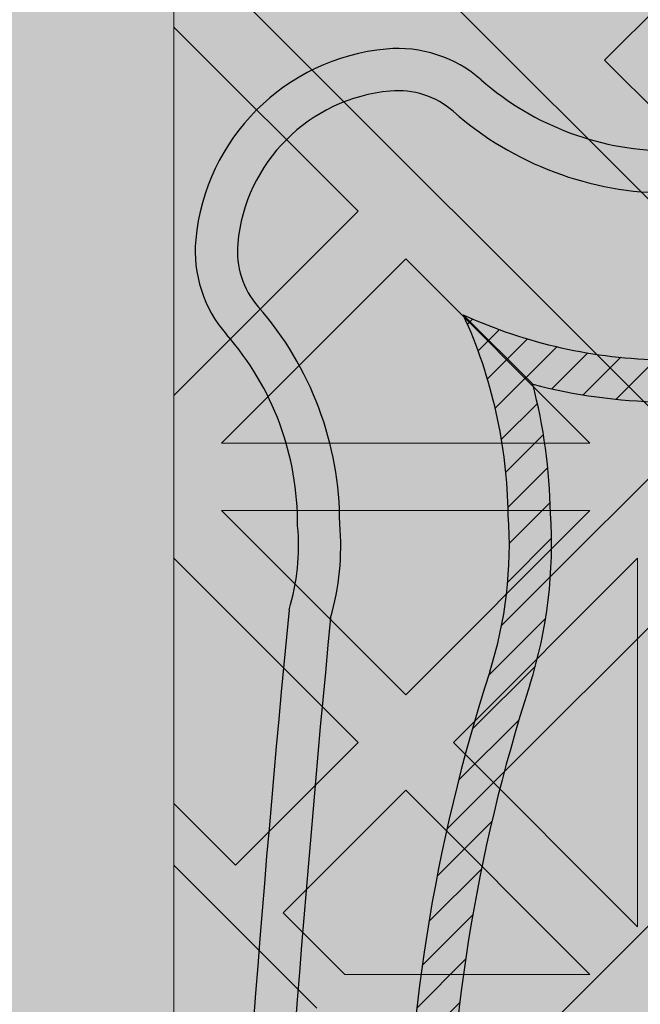
# Model space of a CAD drawing. Units: inches. Extents: x 844 to 2234, y 346 to 1084.
# Tile 58 of 93: x 1864.294 to 1866.641, y 706.48 to 710.205. Entities that reach past the tile are written whole.
import ezdxf

# ---------------------------------------------------------------- set-up
doc = ezdxf.new("R2010")
doc.units = ezdxf.units.IN
doc.header["$MEASUREMENT"] = 0
doc.layers.add('furniture', color=8, linetype='Continuous', lineweight=18)
doc.layers.add('RA-AP-01$0$INT', color=35, linetype='Continuous', lineweight=5)
doc.layers.add('RA-AP-01$0$FURN', color=3, linetype='Continuous')
doc.layers.add('RA-AP-01$0$WOOD', color=64, linetype='Continuous')

# ---------------------------------------------------------------- blocks, each defined once
blk = doc.blocks.new('A$C18D01794')
at = {"layer": 'RA-AP-01$0$INT'}
blk.add_hatch(color=256, dxfattribs=at).paths.add_polyline_path([(4.505206456958071, -7.906712009588039), (5.305206456958072, -7.906712009588039), (5.305206456958072, -7.106712009588038), (5.255206456951893, -7.106712009588036), (5.25520645694868, -7.856712009570104), (4.555206456959269, -7.856712009588616), (4.555206456956052, -7.106712009588038), (4.505206456958073, -7.106712009588038)])
h = blk.add_hatch(color=256, dxfattribs=at)
h.paths.add_polyline_path([(4.585917135068448, -7.856712009587804), (4.614201406330596, -7.856712009587056), (4.668846067270487, -7.802067348644738), (4.723490728212344, -7.856712009584164), (4.771774999457151, -7.856712009582887), (4.826419660396886, -7.80206734864072), (4.862780050090322, -7.838427738332541), (4.844495778842715, -7.856712009580965), (4.862780050090411, -7.856712009580482), (4.905206456960182, -7.814285602707865), (4.947632863832445, -7.856712009578238), (4.965917135079675, -7.856712009577755), (4.947632863831759, -7.838427738330656), (4.983993253523576, -7.802067348637219), (5.038637914464627, -7.856712009575829), (5.08692218571208, -7.856712009574554), (5.141566846649976, -7.802067348634224), (5.196211507589851, -7.856712009571666), (5.224495778822615, -7.856712009570916), (4.905206456953975, -7.537422687702283)])
h.paths.add_polyline_path([(4.895206456956031, -7.575706958950402), (4.895206456958921, -7.684996280828174), (4.840561796018589, -7.630351619890275)], flags=16)
h.paths.add_polyline_path([(4.915206456955638, -7.575706958949956), (4.969851117895509, -7.630351619887399), (4.915206456957609, -7.684996280827732)], flags=16)
h.paths.add_polyline_path([(4.826419660395175, -7.644493755514321), (4.881064321335613, -7.699138416452331), (4.771774999456703, -7.69913841645522)], flags=16)
h.paths.add_polyline_path([(4.983993253519558, -7.644493755510815), (5.038637914460456, -7.699138416449285), (4.929348592581548, -7.69913841645126)], flags=16)
h.paths.add_polyline_path([(4.881064321336025, -7.719138416452334), (4.826419660397532, -7.773783077393256), (4.771774999457062, -7.719138416455217)], flags=16)
h.paths.add_polyline_path([(4.929348592582019, -7.71913841645126), (5.038637914460982, -7.719138416449284), (4.983993253522945, -7.773783077389749)], flags=16)
h.paths.add_polyline_path([(4.895206456960191, -7.733280552075633), (4.895206456962115, -7.806001331460164), (4.876922185715016, -7.824285602708492), (4.840561796021581, -7.787925213016675)], flags=16)
h.paths.add_polyline_path([(4.915206456958487, -7.733280552075187), (4.969851117899527, -7.787925213013798), (4.933490728206909, -7.824285602708034), (4.9152064569598, -7.806001331461736)], flags=16)
h.paths.add_polyline_path([(4.757632863832376, -7.733280552079264), (4.812277524772842, -7.787925213017304), (4.757632863834348, -7.842569873958233)], flags=16)
h.paths.add_polyline_path([(4.737632863832376, -7.73328055207979), (4.737632863834348, -7.842569873958701), (4.682988202893906, -7.787925213020692)], flags=16)
h.paths.add_polyline_path([(5.05278005008503, -7.733280552072701), (5.052780050087917, -7.842569873951664), (4.998135389146995, -7.787925213013169)], flags=16)
h.paths.add_polyline_path([(5.072780050085024, -7.733280552072333), (5.127424711025931, -7.787925213010806), (5.072780050087916, -7.842569873951244)], flags=16)
h.paths.add_polyline_path([(4.935917135072783, -7.506712009583784), (5.255206456948811, -7.826001331459767), (5.255206456948932, -7.797717060211899), (5.200561796010279, -7.743072399273238), (5.255206456949403, -7.688427738334128), (5.25520645694961, -7.640143467086677), (5.200561796009787, -7.585498806146837), (5.236922185702417, -7.549138416454212), (5.255206456949919, -7.56742268770172), (5.255206456949998, -7.549138416454178), (5.212780050078687, -7.506712009583814), (5.25520645695036, -7.464285602712145), (5.255206456950438, -7.446001331464763), (5.236922185702424, -7.464285602712779), (5.200561796009796, -7.427925213020149), (5.255206456950753, -7.373280552079203), (5.25520645695096, -7.324996280834394), (5.200561796010322, -7.270351619893748), (5.255206456951428, -7.215706958952649), (5.255206456951547, -7.187422687705071)])
h.paths.add_polyline_path([(5.042988202883395, -7.42792521302065), (5.097632863823085, -7.373280552080975), (5.097632863822622, -7.482569873959883)], flags=16)
h.paths.add_polyline_path([(5.028846067259663, -7.442067348644384), (5.083490728198774, -7.496712009583504), (4.974201406321001, -7.496712009583035)], flags=16)
h.paths.add_polyline_path([(5.117632863823087, -7.37328055208089), (5.172277524762331, -7.42792521302015), (5.11763286382262, -7.482569873959851)], flags=16)
h.paths.add_polyline_path([(5.08349072819877, -7.516712009582191), (5.028846067259652, -7.571356670521302), (4.974201406320998, -7.516712009582638)], flags=16)
h.paths.add_polyline_path([(5.131774999446817, -7.35913841645716), (5.186419660386065, -7.413783077396415), (5.241064321325782, -7.359138416456712)], flags=17)
h.paths.add_polyline_path([(5.131774999446228, -7.496712009583703), (5.186419660386065, -7.442067348643883), (5.222780050079488, -7.478427738337313), (5.204495778832781, -7.496712009584014)], flags=16)
h.paths.add_polyline_path([(5.097632863822613, -7.530854145205813), (5.097632863823061, -7.640143467084723), (5.042988202883383, -7.585498806145032)], flags=16)
h.paths.add_polyline_path([(5.131774999446899, -7.339138416457162), (5.241064321325809, -7.339138416456712), (5.186419660386591, -7.284493755517479)], flags=17)
h.paths.add_polyline_path([(5.131774999446226, -7.516712009581999), (5.204495778830767, -7.516712009581702), (5.22278005007868, -7.534996280829206), (5.186419660386049, -7.571356670521828)], flags=16)
h.paths.add_polyline_path([(5.11763286382262, -7.530854145205852), (5.17227752476232, -7.585498806145562), (5.117632863823064, -7.64014346708481)], flags=16)
h.paths.add_polyline_path([(5.186419660386069, -7.599640941770585), (5.241064321325754, -7.654285602710281), (5.131774999446791, -7.654285602709814)], flags=16)
h.paths.add_polyline_path([(5.131774999446872, -7.674285602709813), (5.24106432132578, -7.674285602710282), (5.186419660386554, -7.728930263649504)], flags=16)
h.paths.add_polyline_path([(5.255206456951811, -7.126001331467467), (5.255206456951895, -7.106712009588038), (4.555206456956052, -7.106712009588038), (4.555206456956136, -7.12600133146746), (4.905206456953973, -7.476001331465289)])
h.paths.add_polyline_path([(4.983993253513404, -7.368930263651977), (4.92934859257295, -7.314285602713969), (5.03863791445186, -7.314285602711063)], flags=16)
h.paths.add_polyline_path([(4.969851117889988, -7.383072399276016), (4.915206456952556, -7.437717060215906), (4.915206456949648, -7.328427738338133)], flags=16)
h.paths.add_polyline_path([(4.929348592572535, -7.294285602713971), (4.983993253511019, -7.239640941773039), (5.038637914451496, -7.294285602711065)], flags=16)
h.paths.add_polyline_path([(5.052780050074912, -7.280143467087016), (4.998135389134438, -7.225498806148989), (5.052780050072919, -7.170854145208052)], flags=16)
h.paths.add_polyline_path([(5.07278005007491, -7.280143467086489), (5.072780050072918, -7.170854145207579), (5.127424711013374, -7.225498806145578)], flags=16)
h.paths.add_polyline_path([(4.89520645695295, -7.437717060216355), (4.840561796013067, -7.383072399278919), (4.895206456950961, -7.328427738338582)], flags=16)
h.paths.add_polyline_path([(4.915206456948365, -7.280143467090674), (4.915206456946434, -7.207422687704125), (4.933490728192729, -7.18913841645701), (4.969851117886972, -7.225498806149623)], flags=16)
h.paths.add_polyline_path([(4.881064321327021, -7.314285602715054), (4.82641966038902, -7.368930263655506), (4.771774999448108, -7.314285602717047)], flags=16)
h.paths.add_polyline_path([(4.895206456950073, -7.280143467091125), (4.840561796009022, -7.225498806152518), (4.876922185700835, -7.18913841645908), (4.895206456948749, -7.207422687706589)], flags=16)
h.paths.add_polyline_path([(4.983993253510392, -7.211356670525576), (4.947632863816944, -7.174996280833758), (4.965917135064043, -7.156712009585847), (5.038637914448995, -7.156712009584522)], flags=16)
h.paths.add_polyline_path([(4.881064321326543, -7.294285602715056), (4.771774999447578, -7.294285602717046), (4.826419660385607, -7.239640941776569)], flags=16)
h.paths.add_polyline_path([(4.905206456946447, -7.19913841645844), (4.862780050074785, -7.156712009587725), (4.947632863816685, -7.156712009586302)], flags=16)
h.paths.add_polyline_path([(5.14156684663679, -7.211356670521528), (5.086922185696452, -7.156712009583639), (5.196211507574223, -7.156712009581651)], flags=16)
h.paths.add_polyline_path([(4.8264196603837, -7.211356670529104), (4.771774999442643, -7.156712009590501), (4.8444957788276, -7.156712009588568), (4.862780050075511, -7.17499628083566)], flags=16)
h.paths.add_polyline_path([(4.812277524760289, -7.225498806153156), (4.757632863822258, -7.28014346709363), (4.757632863819352, -7.170854145214669)], flags=16)
h.paths.add_polyline_path([(4.73763286382226, -7.280143467093997), (4.682988202881349, -7.22549880615554), (4.737632863819352, -7.170854145215086)], flags=16)
h.paths.add_polyline_path([(4.723490728195188, -7.156712009591787), (4.668846067257299, -7.211356670532127), (4.614201406317417, -7.156712009594693)], flags=16)
h.paths.add_polyline_path([(4.597632863829262, -7.506712009583814), (4.555206456957951, -7.54913841645418), (4.555206456958029, -7.56742268770172), (4.573490728205535, -7.549138416454212), (4.609851117898167, -7.585498806146839), (4.555206456958338, -7.640143467086675), (4.555206456958546, -7.688427738334125), (4.60985111789767, -7.743072399273238), (4.555206456959015, -7.797717060211899), (4.555206456959138, -7.826001331459767), (4.874495778835167, -7.506712009583786), (4.5552064569564, -7.187422687705062), (4.555206456956523, -7.215706958952644), (4.609851117897629, -7.270351619893746), (4.555206456956988, -7.324996280834396), (4.555206456957198, -7.373280552079195), (4.609851117898153, -7.427925213020147), (4.573490728205528, -7.464285602712779), (4.555206456957507, -7.446001331464756), (4.555206456957585, -7.464285602712143)])
h.paths.add_polyline_path([(4.712780050085332, -7.482569873959882), (4.712780050084863, -7.373280552080972), (4.767424711024555, -7.42792521302065)], flags=16)
h.paths.add_polyline_path([(4.726922185709173, -7.496712009583504), (4.781566846648288, -7.442067348644384), (4.836211507586949, -7.496712009583033)], flags=16)
h.paths.add_polyline_path([(4.692780050085327, -7.482569873959851), (4.638135389145619, -7.427925213020149), (4.692780050084865, -7.373280552080892)], flags=16)
h.paths.add_polyline_path([(4.726922185709182, -7.516712009582191), (4.836211507586949, -7.51671200958264), (4.7815668466483, -7.571356670521304)], flags=16)
h.paths.add_polyline_path([(4.678637914461726, -7.496712009583706), (4.605917135075169, -7.496712009584014), (4.587632863828464, -7.478427738337311), (4.623993253521887, -7.442067348643881)], flags=16)
h.paths.add_polyline_path([(4.712780050085336, -7.530854145205816), (4.767424711024568, -7.585498806145034), (4.71278005008489, -7.640143467084724)], flags=16)
h.paths.add_polyline_path([(4.678637914461726, -7.516712009582001), (4.623993253521899, -7.571356670521829), (4.587632863829271, -7.534996280829206), (4.605917135077185, -7.5167120095817)], flags=16)
h.paths.add_polyline_path([(4.692780050085336, -7.530854145205848), (4.692780050084889, -7.64014346708481), (4.638135389145632, -7.585498806145562)], flags=16)
h.paths.add_polyline_path([(4.623993253521885, -7.413783077396415), (4.678637914461131, -7.359138416457161), (4.56934859258217, -7.359138416456712)], flags=17)
h.paths.add_polyline_path([(4.623993253521901, -7.599640941770568), (4.678637914461158, -7.654285602709814), (4.569348592582195, -7.654285602710281)], flags=16)
h.paths.add_polyline_path([(4.678637914461051, -7.339138416457162), (4.623993253521361, -7.284493755517479), (4.569348592582143, -7.339138416456712)], flags=17)
h.paths.add_polyline_path([(4.678637914461076, -7.674285602709813), (4.623993253521399, -7.728930263649504), (4.569348592582167, -7.674285602710281)], flags=16)
h = blk.add_hatch(color=256, dxfattribs=at)
h.paths.add_polyline_path([(4.905206456954232, -7.537422687702028), (4.874495778835232, -7.506712009583718), (4.555206456959138, -7.826001331459766), (4.555206456959269, -7.856712009588616), (4.585917135068449, -7.856712009587804)])
h.paths.add_polyline_path([(4.935917135072152, -7.506712009583152), (4.905206456953497, -7.537422687701806), (5.224495778822614, -7.856712009570917), (5.255206456948681, -7.856712009570104), (5.255206456948813, -7.826001331459768)])
h.paths.add_polyline_path([(5.255206456951549, -7.18742268770507), (5.255206456951813, -7.126001331467461), (4.905206456953563, -7.476001331465701), (4.935917135072559, -7.506712009584006)])
h.paths.add_polyline_path([(4.874495778835167, -7.506712009583785), (4.905206456953818, -7.476001331465132), (4.555206456956135, -7.126001331467458), (4.555206456956399, -7.187422687705064)])
h = blk.add_hatch(color=256, dxfattribs=at)
h.paths.add_polyline_path([(4.781566846647504, -7.442067348645805), (4.836211507586161, -7.496712009584463), (4.726922185708388, -7.496712009584918)])
h.paths.add_polyline_path([(4.836211507586161, -7.516712009584068), (4.781566846647504, -7.571356670522723), (4.726922185708388, -7.516712009583606)])
h.paths.add_polyline_path([(4.76742471102377, -7.585498806146453), (4.712780050084083, -7.640143467086137), (4.712780050084542, -7.530854145207227)])
h.paths.add_polyline_path([(4.692780050084544, -7.530854145207257), (4.692780050084084, -7.64014346708622), (4.638135389144834, -7.585498806146965)])
h.paths.add_polyline_path([(4.678637914460932, -7.516712009583407), (4.623993253521102, -7.571356670523233), (4.587632863827676, -7.53499628082981), (4.605917135074382, -7.516712009583104)])
h.paths.add_polyline_path([(4.573490728204743, -7.54913841645434), (4.60985111789737, -7.585498806146969), (4.555206456957541, -7.640143467086797), (4.555206456957237, -7.567422687701846)])
h.paths.add_polyline_path([(4.623993253521098, -7.599640941770699), (4.67863791446035, -7.654285602709951), (4.56934859258139, -7.654285602710407)])
h.paths.add_polyline_path([(4.678637914460275, -7.67428560270995), (4.623993253520583, -7.728930263649637), (4.56934859258136, -7.674285602710405)])
h.paths.add_polyline_path([(4.609851117896854, -7.743072399273369), (4.555206456958196, -7.797717060212026), (4.555206456957738, -7.688427738334254)])
h.paths.add_polyline_path([(4.597632863828475, -7.506712009583301), (4.555206456957283, -7.549138416454495), (4.555206456956805, -7.464285602712587)])
h.paths.add_polyline_path([(4.678637914460932, -7.496712009585113), (4.605917135076396, -7.496712009585417), (4.587632863828479, -7.478427738337913), (4.623993253521104, -7.442067348645284)])
h.paths.add_polyline_path([(4.692780050084091, -7.373280552082301), (4.692780050084548, -7.482569873961267), (4.638135389144834, -7.427925213021552)])
h.paths.add_polyline_path([(4.767424711023772, -7.427925213022072), (4.712780050084545, -7.48256987396129), (4.712780050084089, -7.373280552082384)])
h.paths.add_polyline_path([(4.67863791446036, -7.359138416457298), (4.623993253521105, -7.41378307739655), (4.569348592581399, -7.35913841645684)])
h.paths.add_polyline_path([(4.609851117897371, -7.427925213020278), (4.573490728204743, -7.464285602712907), (4.555206456957237, -7.446001331465401), (4.555206456957548, -7.373280552080448)])
h.paths.add_polyline_path([(4.623993253520596, -7.284493755517612), (4.67863791446028, -7.339138416457299), (4.569348592581367, -7.339138416456838)])
h.paths.add_polyline_path([(4.609851117896867, -7.270351619893878), (4.555206456957749, -7.324996280832994), (4.55520645695821, -7.21570695895522)])
h = blk.add_hatch(color=256, dxfattribs=at)
h.paths.add_polyline_path([(4.969851117891331, -7.630351619889621), (4.915206456952669, -7.575706958950966), (4.915206456952222, -7.684996280828739)])
h.paths.add_polyline_path([(4.895206456953064, -7.575706958950968), (4.840561796014413, -7.630351619889628), (4.895206456953533, -7.684996280828741)])
h.paths.add_polyline_path([(4.826419660390684, -7.644493755513362), (4.771774999451003, -7.699138416453052), (4.881064321329913, -7.699138416452587)])
h.paths.add_polyline_path([(4.881064321329884, -7.719138416452585), (4.771774999450921, -7.719138416453052), (4.82641966039018, -7.773783077392298)])
h.paths.add_polyline_path([(4.895206456953734, -7.733280552076196), (4.840561796013912, -7.787925213016031), (4.876922185707337, -7.824285602709455), (4.895206456954043, -7.806001331462747)])
h.paths.add_polyline_path([(4.862780050082808, -7.838427738332388), (4.826419660390178, -7.802067348639763), (4.771774999450351, -7.856712009579595), (4.844495778835303, -7.856712009579895)])
h.paths.add_polyline_path([(4.812277524766446, -7.787925213016036), (4.757632863827191, -7.733280552076788), (4.757632863826741, -7.842569873955747)])
h.paths.add_polyline_path([(4.737632863827191, -7.733280552076863), (4.682988202887508, -7.787925213016558), (4.737632863826743, -7.842569873955778)])
h.paths.add_polyline_path([(4.668846067263777, -7.802067348640287), (4.614201406325123, -7.856712009578949), (4.723490728202894, -7.856712009579402)])
h.paths.add_polyline_path([(4.905206456953846, -7.814285602708654), (4.862780050082654, -7.856712009579847), (4.947632863824561, -7.85671200958032)])
h.paths.add_polyline_path([(4.915206456952028, -7.733280552076195), (4.91520645695173, -7.806001331460731), (4.933490728199234, -7.824285602708648), (4.96985111789186, -7.787925213016022)])
h.paths.add_polyline_path([(5.038637914454841, -7.719138416453029), (4.929348592575874, -7.71913841645258), (4.983993253515593, -7.773783077392289)])
h.paths.add_polyline_path([(4.983993253515065, -7.644493755513352), (4.929348592575849, -7.699138416452582), (5.038637914454755, -7.699138416453031)])
h.paths.add_polyline_path([(5.052780050079843, -7.73328055207676), (4.998135389140595, -7.787925213016018), (5.052780050080309, -7.842569873955721)])
h.paths.add_polyline_path([(4.983993253516868, -7.802067348639752), (4.947632863824241, -7.838427738332383), (4.965917135071747, -7.856712009579888), (5.038637914456701, -7.856712009579572)])
h.paths.add_polyline_path([(5.127424711019533, -7.787925213016519), (5.072780050079843, -7.733280552076838), (5.07278005008031, -7.842569873955751)])
h.paths.add_polyline_path([(5.141566846643269, -7.802067348640248), (5.086922185704154, -7.85671200957937), (5.196211507581929, -7.856712009578901)])
for p, q in [((4.555206456956052, -7.106712009588036), (4.555206456959269, -7.856712009588616)), ((4.55520645695807, -7.464285602712626), (4.555206456957598, -7.549138416454534)), ((4.597632863829264, -7.506712009583814), (4.555206456957598, -7.549138416454534)), ((4.874495778835167, -7.506712009583786), (4.555206456959136, -7.826001331459769)), ((4.605917135074869, -7.516712009584017), (4.587632863829269, -7.534996280829206)), ((4.605917135076771, -7.5167120095817), (4.678637914461723, -7.516712009581999)), ((4.678637914461723, -7.516712009581999), (4.623993253521898, -7.571356670521829)), ((4.692780050085336, -7.530854145205847), (4.638135389145632, -7.585498806145562)), ((4.692780050084889, -7.64014346708481), (4.692780050085336, -7.530854145205847)), ((4.623993253521899, -7.571356670521829), (4.587632863829269, -7.534996280829206)), ((4.905206456953975, -7.537422687702283), (4.585917135071132, -7.856712009585121)), ((4.555206456958031, -7.56742268770172), (4.573490728205535, -7.549138416454212)), ((4.609851117898167, -7.585498806146839), (4.573490728205535, -7.549138416454214)), ((4.555206456958033, -7.56742268770172), (4.555206456958345, -7.640143467086671)), ((4.555206456958345, -7.640143467086671), (4.609851117898167, -7.585498806146837)), ((4.692780050084889, -7.64014346708481), (4.638135389145632, -7.585498806145562)), ((4.569348592582195, -7.654285602710281), (4.623993253521901, -7.599640941770568)), ((4.678637914461158, -7.654285602709814), (4.623993253521901, -7.599640941770568)), ((4.678637914461158, -7.654285602709814), (4.569348592582195, -7.654285602710281)), ((4.569348592582168, -7.674285602710281), (4.623993253521399, -7.728930263649504)), ((4.678637914461078, -7.674285602709813), (4.569348592582168, -7.674285602710281)), ((4.6239932535214, -7.728930263649502), (4.678637914461078, -7.674285602709813)), ((4.555206456958551, -7.68842773833413), (4.60985111789767, -7.743072399273238)), ((4.682988202893908, -7.78792521302069), (4.737632863832376, -7.733280552079792)), ((4.555206456959017, -7.797717060211899), (4.60985111789767, -7.743072399273238)), ((4.737632863834348, -7.842569873958701), (4.682988202893906, -7.787925213020692))]:
    blk.add_line(p, q, dxfattribs=at)
blk = doc.blocks.new('A$C32926AE1')
at = {"layer": 'RA-AP-01$0$WOOD'}
h = blk.add_hatch(color=256, dxfattribs=at)
h.dxf.hatch_style = 1
h.paths.add_polyline_path([(5.157430609644524, 4.573483066760929, -0.1009492694046607), (5.155401577623758, 4.593365984175333, -0.1842662638101597), (5.172249623284174, 4.638795604568598, 0.2056608120311276), (5.179560981299304, 4.661316324430096, 0.3614336704623542), (5.134352340494423, 4.706524965234944, 0.2056608120311297), (5.111831620632933, 4.699213607219793, -0.1842662638101113), (5.066402000239693, 4.682365561559342, -0.1055311479399994), (5.045656153913092, 4.68467289944697, 0.1567636581983829), (4.763886414745334, 4.684672899446966, -0.1055311479399895), (4.743140568418733, 4.68236556155934, -0.1842662638100833), (4.6977109480255, 4.69921360721979, 0.2056608120302612), (4.675190228164109, 4.706524965234949, 0.3614336704708441), (4.629981587358889, 4.66131632442871, 0.2056608120245944), (4.637292945374126, 4.638795604567974, -0.1842662638101024), (4.654140991034615, 4.59336598417475, -0.1009492694055169), (4.652111959013835, 4.573483066760181, 0.021410119221476), (4.629748025606143, 4.156712009541676, 0.0214101192214795), (4.652111959013809, 3.739940952323101, -0.1009492694059586), (4.654140991034615, 3.720058034908448, -0.1842662638100975), (4.637292945374126, 3.674628414515226, 0.2056608120245705), (4.629981587358889, 3.652107694654492, 0.3614336704708879), (4.675190228164113, 3.606899053848249, 0.2056608120302384), (4.697710948025501, 3.614210411863408, -0.1842662638100995), (4.743140568418738, 3.63105845752386, -0.1055311479402541), (4.763886414745388, 3.628751119636215, 0.1567636581983776), (5.045656153913137, 3.628751119636244, -0.1055311479397538), (5.066402000239692, 3.631058457523857, -0.1842662638101067), (5.111831620632931, 3.614210411863407, 0.2056608120310924), (5.134352340494417, 3.606899053848256, 0.3614336704624001), (5.179560981299307, 3.652107694653103, 0.2056608120311314), (5.172249623284175, 3.6746284145146, -0.1842662638101402), (5.155401577623758, 3.72005803490786, -0.1009492694051366), (5.15743060964455, 3.739940952322354, 0.0214101192215073), (5.179794543052287, 4.156712009541468, 0.0214101192215252)])
h.paths.add_polyline_path([(4.639748609479751, 4.156712009541513, 0.0213537860821624), (4.661970494867118, 3.741887061152232, -0.094075836301374), (4.664143710413708, 3.7196126951003, -0.1824818158568985), (4.644813765429836, 3.668037719127816, 0.2056608120245319), (4.639939526753007, 3.653023905887301, 0.3614336704710246), (4.676106439397173, 3.616856993242342, 0.2056608120302234), (4.691120252638095, 3.621731231919122, -0.1824818158602558), (4.742695228611606, 3.641061176902986, -0.1029891339458722), (4.766991894714349, 3.638256818950944, 0.156709409989566), (5.042550673941472, 3.638256818950105, -0.102989133958497), (5.066847340047078, 3.641061176902949, -0.1824818158594995), (5.118422316020358, 3.621731231919103, 0.2056608120311416), (5.133436129261316, 3.616856993242346, 0.3614336704621468), (5.169603041905217, 3.653023905886178, 0.2056608120310986), (5.164728803228477, 3.668037719127177, -0.1824818158565612), (5.145398858244737, 3.719612695099578, -0.0940758363009313), (5.147572073791232, 3.741887061151398, 0.0213537860822023), (5.169793959178681, 4.156712009541451, 0.0213537860822226), (5.147572073791203, 4.571536957931898, -0.0940758363005034), (5.145398858244737, 4.59381132398362, -0.1824818158565587), (5.164728803228476, 4.645386299956021, 0.2056608120311045), (5.169603041905216, 4.66040011319702, 0.3614336704621845), (5.133436129261313, 4.696567025840856, 0.2056608120310773), (5.118422316020359, 4.691692787164098, -0.182481815859508), (5.066847340047078, 4.67236284218025, -0.1029891339584606), (5.04255067394148, 4.675167200133092, 0.156709409989566), (4.766991894714357, 4.675167200132257, -0.1029891339458842), (4.742695228611611, 4.672362842180213, -0.1824818158602725), (4.691120252638095, 4.691692787164077, 0.2056608120302152), (4.676106439397174, 4.696567025840858, 0.3614336704710363), (4.639939526753005, 4.660400113195899, 0.2056608120245495), (4.644813765429837, 4.645386299955384, -0.1824818158568934), (4.664143710413708, 4.593811323982902, -0.0940758363009187), (4.661970494867149, 4.571536957931074, 0.021353786082177)], flags=16)
h.paths.add_polyline_path([(5.129794543052235, 4.432167055276933, -0.0141661062790638), (5.130152669293814, 4.156927903047693, -0.0141661062790647), (5.129794543052234, 3.881688750818433, -0.0785247771143638), (5.10979738006795, 3.755143611847103, 0.0945969212073497), (5.105408519571111, 3.717898134952927, 0.1043170707844957), (5.116074640131521, 3.670385395016088, 0.1043170707864965), (5.068561900193738, 3.681051515576561, 0.09459692119553), (5.031316423304057, 3.676662655080835, -0.1580239521427272), (4.778226145355827, 3.676662655080367, 0.0945969211986668), (4.740980668464973, 3.681051515576592, 0.1043170707882822), (4.693467928526415, 3.670385395015844, 0.1043170707867916), (4.704134049087309, 3.717898134953662, 0.0945969211972894), (4.69974518859162, 3.755143611844042, -0.0785247771163196), (4.679748025606343, 3.881688750818406, -0.0141661062790663), (4.679389899364763, 4.156927903047693, -0.0141661062790672), (4.679748025606343, 4.432167055276998, -0.0785247771163064), (4.699745188591625, 4.55871219425134, 0.094596921197333), (4.704134049087308, 4.595957671141738, 0.1043170707867205), (4.693467928526416, 4.643470411079523, 0.1043170707882628), (4.740980668464965, 4.632804290518776, 0.0945969211988114), (4.778226145355874, 4.637193151015016, -0.158023952142669), (5.031316423304015, 4.637193151014546, 0.0945969211956361), (5.068561900193736, 4.632804290518806, 0.1043170707864979), (5.11607464013152, 4.643470411079278, 0.1043170707844617), (5.105408519571112, 4.595957671142455, 0.0945969212074597), (5.109797380067959, 4.558712194248236, -0.0785247771143467)], flags=0)
h.paths.add_polyline_path([(5.119794532311105, 4.432259799204851, -0.0142000800617244), (5.120156169157484, 4.156927903047701, -0.0142000800617277), (5.119794532311105, 3.881596006890482, -0.0784894509520253), (5.100273383573699, 3.758192358677797, 0.0940138827242913), (5.095413455884425, 3.717477693979438, 0.0606271852308753), (5.099615656341024, 3.686844378806616, 0.0606271852322524), (5.068982341167493, 3.691046579263239, 0.0940138827010453), (5.028267676478798, 3.686186651576848, -0.1580706864508061), (4.781274892180912, 3.686186651576435, 0.0940138827026903), (4.740560227491556, 3.691046579263279, 0.0606271852339895), (4.709926912317155, 3.686844378806508, 0.0606271852329405), (4.714129112773991, 3.717477693980356, 0.094013882701304), (4.709269185087677, 3.758192358669163, -0.0784894509577193), (4.689748036347473, 3.881596006890469, -0.014200080061729), (4.689386399501094, 4.156927903047709, -0.0142000800617217), (4.689748036347473, 4.432259799204808, -0.078489450957724), (4.709269185087651, 4.555663447426125, 0.0940138827014585), (4.714129112773992, 4.596378112114996, 0.0606271852329731), (4.709926912317154, 4.62701142728886, 0.0606271852340196), (4.74056022749157, 4.622809226832087, 0.0940138827024997), (4.781274892180847, 4.627669154518912, -0.1580706864508359), (5.028267676478777, 4.627669154518526, 0.0940138827010946), (5.068982341167492, 4.622809226832129, 0.060627185232254), (5.099615656341024, 4.627011427288751, 0.0606271852308727), (5.095413455884425, 4.59637811211593, 0.0940138827241088), (5.100273383573675, 4.555663447417647, -0.0784894509520978)], flags=0)
h.paths.add_polyline_path([(5.06978912287499, 4.430218106756144, -0.014241683694547), (5.070173729147532, 4.156927903047672, -0.0142416836945458), (5.06978912287499, 3.883637699339223, -0.0800609523125196), (5.052662118612511, 3.773463122773442, 0.0526421978001116), (5.04590916754064, 3.740550867606997, 0.0526421977992423), (5.012996912374707, 3.73379791653534, -0.1583028414718258), (4.796545656286308, 3.73379791653451, 0.0526421978034211), (4.763633401117837, 3.740550867607021, 0.0526421978018622), (4.756880450045755, 3.773463122774558, -0.0800609523117106), (4.739753445783639, 3.883637699339268, -0.0142416836945435), (4.739368839511098, 4.156927903047671, -0.0142416836945477), (4.739753445783639, 4.430218106756155, -0.0800609523116345), (4.75688045004574, 4.540392683320762, 0.052642197801941), (4.763633401117837, 4.573304938488346, 0.0526421978035071), (4.796545656286361, 4.580057889560873, -0.1583028414717561), (5.012996912374669, 4.580057889560039, 0.0526421977993048), (5.04590916754064, 4.57330493848837, 0.0526421978002057), (5.052662118612529, 4.540392683321868, -0.080060952312477)], flags=0)
h.paths.add_polyline_path([(5.049789715110557, 4.43038092723357, -0.0143097550741839), (5.05018085590259, 4.156927903047715, -0.0143097550741854), (5.049789715110558, 3.883474878861827, -0.0800685599149176), (5.03362098255317, 3.779581877367999, 0.0306258898956367), (5.028241146483733, 3.758218888663947, 0.0306258898977031), (5.006878157778253, 3.75283905259408, -0.1583983521624096), (4.802664410878162, 3.752839052594731, 0.0306258898946014), (4.781301422174808, 3.758218888663924, 0.0306258898967912), (4.775921586105202, 3.779581877368794, -0.080068559914251), (4.759752853548071, 3.883474878861786, -0.0143097550741854), (4.759361712756037, 4.156927903047671, -0.0143097550741854), (4.759752853548071, 4.430380927233557, -0.0800685599142479), (4.775921586105193, 4.534273928726546, 0.0306258898968306), (4.781301422174808, 4.555636917431444, 0.0306258898945754), (4.802664410878143, 4.561016753500631, -0.1583983521624168), (5.006878157778244, 4.561016753501291, 0.0306258898977177), (5.028241146483733, 4.555636917431421, 0.0306258898958182), (5.03362098255321, 4.534273928727244, -0.080068559914796)], flags=0)
h.paths.add_polyline_path([(4.999766070382627, 4.428171244713864, -0.0143443147609634), (5.000198441819402, 4.156927903047689, -0.0143443147609612), (4.999766070382627, 3.885684561381556, -0.0784641635803329), (4.987356730658798, 3.799103304488872, -0.1506053783831347), (4.822185837999821, 3.79910330448882, -0.0784641635803318), (4.809776498276007, 3.885684561381509, -0.014344314760963), (4.809344126839227, 4.156927903047677, -0.0143443147609645), (4.809776498276007, 4.428171244713873, -0.0784641635803192), (4.822185837999822, 4.514752501606549, -0.1506053783831338), (4.987356730658798, 4.514752501606494, -0.078464163580285)], flags=0)
h.paths.add_polyline_path([(4.979755254238824, 4.42764379880488, -0.0143772539198268), (4.980205517789977, 4.156927903047693, -0.0143772539198275), (4.979755254238824, 3.886212007290489, -0.0689242507424422), (4.971183264704897, 3.815276770442801, -0.1296645318904179), (4.838359303953726, 3.815276770442746, -0.0689242507424186), (4.829787314419809, 3.886212007290419, -0.0143772539198292), (4.829337050868653, 4.156927903047653, -0.0143772539198325), (4.829787314419809, 4.427643798804946, -0.0689242507424211), (4.838359303953725, 4.498579035652621, -0.1296645318904187), (4.971183264704897, 4.498579035652565, -0.0689242507424401)], flags=0)
h = blk.add_hatch(color=256, dxfattribs=at)
h.dxf.hatch_style = 1
h.paths.add_polyline_path([(5.145398858244737, 4.59381132398362, -0.1824818158565616), (5.164728803228476, 4.645386299956021, 0.2056608120311045), (5.169603041905216, 4.66040011319702, 0.3614336704621845), (5.133436129261313, 4.696567025840856, 0.2056608120310773), (5.118422316020359, 4.691692787164098, -0.182481815859508), (5.066847340047078, 4.67236284218025, -0.1029891339584606), (5.04255067394148, 4.675167200133092, 0.156709409989566), (4.766991894714357, 4.675167200132257, -0.1029891339458842), (4.742695228611611, 4.672362842180213, -0.1824818158602725), (4.691120252638095, 4.691692787164077, 0.2056608120302152), (4.676106439397174, 4.696567025840858, 0.3614336704710363), (4.639939526753005, 4.660400113195899, 0.2056608120245495), (4.644813765429837, 4.645386299955384, -0.1824818158568934), (4.664143710413708, 4.593811323982902, -0.0940758363009187), (4.661970494867149, 4.571536957931074, 0.0213537860821772), (4.639748609479751, 4.156712009541507, 0.0213537860821625), (4.661970494867119, 3.741887061152226, -0.0940758363013071), (4.664143710413708, 3.719612695100309, -0.1824818158569294), (4.644813765429836, 3.668037719127816, 0.2056608120245319), (4.639939526753007, 3.653023905887301, 0.3614336704710246), (4.676106439397173, 3.616856993242342, 0.2056608120302234), (4.691120252638095, 3.621731231919122, -0.1824818158602558), (4.742695228611606, 3.641061176902986, -0.1029891339458722), (4.766991894714349, 3.638256818950944, 0.156709409989566), (5.042550673941472, 3.638256818950105, -0.102989133958497), (5.066847340047078, 3.641061176902949, -0.1824818158594995), (5.118422316020358, 3.621731231919103, 0.2056608120311416), (5.133436129261316, 3.616856993242346, 0.3614336704621468), (5.169603041905217, 3.653023905886178, 0.2056608120310986), (5.164728803228477, 3.668037719127177, -0.1824818158565612), (5.145398858244737, 3.719612695099578, -0.0940758363009313), (5.147572073791232, 3.741887061151398, 0.0213537860822023), (5.169793959178681, 4.156712009541451, 0.0213537860822226), (5.147572073791203, 4.571536957931898, -0.0940758363004996)])
h.paths.add_polyline_path([(5.109797380067958, 4.55871219424824, -0.0785247771143472), (5.129794543052234, 4.432167055276936, -0.0141661062790644), (5.130152669293814, 4.156927903047685, -0.014166106279066), (5.129794543052234, 3.881688750818401, -0.0785247771143517), (5.109797380067946, 3.755143611847092, 0.0945969212073132), (5.105408519571111, 3.717898134952929, 0.1043170707844995), (5.116074640131521, 3.670385395016088, 0.1043170707864965), (5.068561900193738, 3.681051515576561, 0.09459692119553), (5.031316423304057, 3.676662655080835, -0.1580239521427272), (4.778226145355827, 3.676662655080367, 0.0945969211986668), (4.740980668464973, 3.681051515576592, 0.1043170707882822), (4.693467928526415, 3.670385395015844, 0.1043170707867916), (4.704134049087309, 3.717898134953662, 0.0945969211972894), (4.69974518859162, 3.755143611844042, -0.0785247771163196), (4.679748025606343, 3.881688750818406, -0.0141661062790663), (4.679389899364763, 4.156927903047693, -0.0141661062790672), (4.679748025606343, 4.432167055276998, -0.0785247771163064), (4.699745188591625, 4.55871219425134, 0.094596921197333), (4.704134049087308, 4.595957671141738, 0.1043170707867205), (4.693467928526416, 4.643470411079523, 0.1043170707882628), (4.740980668464965, 4.632804290518776, 0.0945969211988114), (4.778226145355874, 4.637193151015016, -0.158023952142669), (5.031316423304015, 4.637193151014546, 0.0945969211956361), (5.068561900193736, 4.632804290518806, 0.1043170707864979), (5.11607464013152, 4.643470411079278, 0.1043170707844617), (5.105408519571112, 4.595957671142455, 0.0945969212074504)], flags=16)
h.paths.add_polyline_path([(5.100273383573655, 4.55566344741771, -0.0784894509521388), (5.119794532311105, 4.432259799204852, -0.0142000800617252), (5.120156169157484, 4.156927903047686, -0.014200080061726), (5.119794532311105, 3.881596006890502, -0.0784894509520446), (5.100273383573696, 3.758192358677786, 0.0940138827242721), (5.095413455884425, 3.717477693979436, 0.0606271852308692), (5.099615656341024, 3.686844378806616, 0.0606271852322522), (5.068982341167493, 3.691046579263239, 0.0940138827010453), (5.028267676478798, 3.686186651576848, -0.1580706864508061), (4.781274892180912, 3.686186651576435, 0.0940138827026903), (4.740560227491556, 3.691046579263279, 0.0606271852339895), (4.709926912317155, 3.686844378806508, 0.0606271852329405), (4.714129112773991, 3.717477693980356, 0.094013882701304), (4.709269185087677, 3.758192358669163, -0.0784894509577193), (4.689748036347473, 3.881596006890469, -0.014200080061729), (4.689386399501094, 4.156927903047709, -0.0142000800617217), (4.689748036347473, 4.432259799204808, -0.078489450957724), (4.709269185087651, 4.555663447426125, 0.0940138827014585), (4.714129112773992, 4.596378112114996, 0.0606271852329731), (4.709926912317154, 4.62701142728886, 0.0606271852340196), (4.74056022749157, 4.622809226832087, 0.0940138827024997), (4.781274892180847, 4.627669154518912, -0.1580706864508359), (5.028267676478777, 4.627669154518526, 0.0940138827010946), (5.068982341167492, 4.622809226832129, 0.060627185232254), (5.099615656341024, 4.627011427288751, 0.0606271852308727), (5.095413455884425, 4.59637811211593, 0.094013882723957)], flags=0)
h.paths.add_polyline_path([(5.04590916754064, 4.57330493848837, 0.0526421978002057), (5.052662118612529, 4.540392683321868, -0.0800609523124783), (5.06978912287499, 4.430218106756142, -0.0142416836945469), (5.070173729147532, 4.156927903047672, -0.0142416836945458), (5.06978912287499, 3.883637699339223, -0.0800609523125196), (5.052662118612511, 3.773463122773442, 0.0526421978001116), (5.04590916754064, 3.740550867606997, 0.0526421977992423), (5.012996912374707, 3.73379791653534, -0.1583028414718258), (4.796545656286308, 3.73379791653451, 0.0526421978034211), (4.763633401117837, 3.740550867607021, 0.0526421978018622), (4.756880450045755, 3.773463122774558, -0.0800609523117106), (4.739753445783639, 3.883637699339268, -0.0142416836945435), (4.739368839511098, 4.156927903047671, -0.0142416836945477), (4.739753445783639, 4.430218106756155, -0.0800609523116345), (4.75688045004574, 4.540392683320762, 0.052642197801941), (4.763633401117837, 4.573304938488346, 0.0526421978035071), (4.796545656286361, 4.580057889560873, -0.1583028414717561), (5.012996912374669, 4.580057889560039, 0.0526421977993048)], flags=0)
h.paths.add_polyline_path([(5.028241146483733, 4.555636917431422, 0.0306258898956949), (5.033620982553182, 4.534273928727329, -0.0800685599148649), (5.049789715110557, 4.430380927233569, -0.0143097550741839), (5.05018085590259, 4.156927903047715, -0.0143097550741854), (5.049789715110558, 3.883474878861827, -0.0800685599149176), (5.03362098255317, 3.779581877367999, 0.0306258898956367), (5.028241146483733, 3.758218888663947, 0.0306258898977031), (5.006878157778253, 3.75283905259408, -0.1583983521624096), (4.802664410878162, 3.752839052594731, 0.0306258898946014), (4.781301422174808, 3.758218888663924, 0.0306258898967912), (4.775921586105202, 3.779581877368794, -0.080068559914251), (4.759752853548071, 3.883474878861786, -0.0143097550741854), (4.759361712756037, 4.156927903047671, -0.0143097550741854), (4.759752853548071, 4.430380927233557, -0.0800685599142479), (4.775921586105193, 4.534273928726546, 0.0306258898968306), (4.781301422174808, 4.555636917431444, 0.0306258898945754), (4.802664410878143, 4.561016753500631, -0.1583983521624168), (5.006878157778244, 4.561016753501291, 0.0306258898977174)], flags=0)
h.paths.add_polyline_path([(4.987356730658798, 4.514752501606494, -0.0784641635803018), (4.999766070382627, 4.428171244713845, -0.0143443147609637), (5.000198441819402, 4.156927903047665, -0.0143443147609622), (4.999766070382628, 3.885684561381514, -0.0784641635802952), (4.987356730658797, 3.799103304488872, -0.1506053783831338), (4.822185837999821, 3.799103304488819, -0.0784641635803342), (4.809776498276007, 3.885684561381512, -0.0143443147609628), (4.809344126839227, 4.156927903047676, -0.0143443147609646), (4.809776498276007, 4.428171244713873, -0.0784641635803192), (4.822185837999822, 4.514752501606549, -0.1506053783831338)], flags=0)
h.paths.add_polyline_path([(4.971183264704897, 4.498579035652566, -0.0689242507424384), (4.979755254238824, 4.427643798804883, -0.0143772539198276), (4.980205517789977, 4.15692790304768, -0.0143772539198258), (4.979755254238823, 3.88621200729051, -0.0689242507424628), (4.971183264704897, 3.815276770442801, -0.129664531890417), (4.838359303953726, 3.815276770442746, -0.0689242507424186), (4.829787314419809, 3.886212007290419, -0.0143772539198292), (4.829337050868653, 4.156927903047653, -0.0143772539198325), (4.829787314419809, 4.427643798804946, -0.0689242507424211), (4.838359303953725, 4.498579035652621, -0.1296645318904187)], flags=0)
h = blk.add_hatch(dxfattribs=at)
h.set_pattern_fill('ANSI31', color=256, scale=0.05, style=0)
h.set_pattern_definition([(45, (0, 0), (-0.0044194173824159, 0.0044194173824159), [])])
h.paths.add_polyline_path([(5.130152669293814, 4.156927903047704, 0.0141661062790657), (5.129794543052234, 4.432167055276982, 0.0777827904001433), (5.110168979996553, 4.557559993161921, -0.0976515123401879), (5.105408519571111, 4.595957671142454, -0.1043170707844687), (5.116074640131522, 4.64347041107928), (5.099615656341024, 4.627011427288751, 0.0606271852308727), (5.095413455884425, 4.59637811211593, 0.0940138827241088), (5.100273383573675, 4.555663447417647, -0.0784894509520972), (5.119794532311105, 4.432259799204852, -0.0142000800617252), (5.120156169157484, 4.156927903047686, -0.014200080061726), (5.119794532311105, 3.881596006890502, -0.0784894509520446), (5.100273383573696, 3.758192358677786, 0.0940138827242721), (5.095413455884425, 3.717477693979436, 0.0606271852308692), (5.099615656341024, 3.686844378806616), (5.116074640131519, 3.67038539501609, -0.1043170707844594), (5.105408519571112, 3.717898134952912, -0.0976515123401594), (5.11016897999655, 3.756295812933435, 0.0777827904001654), (5.129794543052234, 3.881688750818409, 0.0141661062790665)])
h.paths.add_polyline_path([(5.030164222210597, 3.676291055149937, -0.0976515123472002), (5.068561900193739, 3.681051515576561, -0.1043170707864927), (5.116074640131521, 3.670385395016088), (5.099615656341024, 3.686844378806616, 0.0606271852322522), (5.068982341167493, 3.691046579263239, 0.0940138827010453), (5.028267676478798, 3.686186651576848, -0.1580706864508061), (4.781274892180912, 3.686186651576435, 0.0940138827026903), (4.740560227491556, 3.691046579263279, 0.0606271852339913), (4.709926912317154, 3.686844378806508), (4.693467928526416, 3.670385395015845, -0.1043170707882796), (4.740980668464973, 3.681051515576592, -0.0976515123427246), (4.779378346446416, 3.676291055150394, 0.156512506893803)])
h.paths.add_polyline_path([(4.689748036347473, 3.881596006890472, -0.014200080061729), (4.689386399501094, 4.156927903047712, -0.0142000800617195), (4.689748036347473, 4.432259799204768, -0.078489450957742), (4.709269185087648, 4.555663447426114, 0.0940138827014821), (4.714129112773992, 4.596378112114995, 0.0606271852329748), (4.709926912317154, 4.62701142728886), (4.693467928526414, 4.643470411079524, -0.1043170707867939), (4.704134049087309, 4.595957671141706, -0.09765151234893), (4.699373588660725, 4.557559993157876, 0.0777827903975372), (4.679748025606343, 4.432167055276987, 0.0141661062790675), (4.679389899364763, 4.156927903047675, 0.0141661062790641), (4.679748025606343, 3.88168875081843, 0.0777827903975637), (4.699373588660724, 3.756295812937497, -0.0976515123490278), (4.704134049087308, 3.717898134953629, -0.1043170707867196), (4.693467928526416, 3.670385395015845), (4.709926912317155, 3.686844378806508, 0.0606271852329413), (4.714129112773991, 3.717477693980357, 0.0940138827013084), (4.709269185087676, 3.758192358669166, -0.0784894509577192)])
h.paths.add_polyline_path([(4.779378346446434, 4.63756475094498, -0.0976515123427943), (4.740980668464964, 4.632804290518776, -0.1043170707882609), (4.693467928526416, 4.643470411079523), (4.709926912317154, 4.62701142728886, 0.0606271852340196), (4.74056022749157, 4.622809226832087, 0.0940138827024997), (4.781274892180847, 4.627669154518912, -0.1580706864508359), (5.028267676478777, 4.627669154518526, 0.0940138827010946), (5.068982341167492, 4.622809226832129, 0.060627185232254), (5.099615656341024, 4.627011427288751), (5.116074640131521, 4.643470411079279, -0.1043170707865022), (5.068561900193735, 4.632804290518806, -0.0976515123475899), (5.030164222210446, 4.637564750945479, 0.1565125068936924)])
h = blk.add_hatch(dxfattribs=at)
h.set_pattern_fill('ANSI32', color=256, scale=0.2, style=0)
h.set_pattern_definition([(45, (0, 0), (-0.0530330085889911, 0.0530330085889911), []), (45, (0.035355339, 0), (-0.0530330085889911, 0.0530330085889911), [])])
h.paths.add_polyline_path([(5.119794532311105, 4.432259799204823, 0.0777015974868765), (5.10065834347252, 4.554469821747928, -0.0968902511992216), (5.095413455884425, 4.596378112115931, -0.060627185230871), (5.099615656341024, 4.627011427288751, -0.060627185232254), (5.068982341167492, 4.622809226832129, -0.0968902512198245), (5.027074050790956, 4.628054114423209, 0.1564657949319105), (4.782468517866163, 4.628054114422785, -0.0968902512152247), (4.740560227491555, 4.622809226832088, -0.0606271852339878), (4.709926912317155, 4.627011427288859, -0.0606271852329413), (4.714129112773991, 4.596378112115011, -0.0968902512205338), (4.708884225182929, 4.554469821738175, 0.0777015974804443), (4.689748036347473, 4.43225979920482, 0.0142000800617215), (4.689386399501094, 4.156927903047726, 0.0142000800617273), (4.689748036347473, 3.88159600689052, 0.077701597480541), (4.708884225182985, 3.759385984357019, -0.096890251220082), (4.714129112773992, 3.717477693980371, -0.0606271852329731), (4.709926912317154, 3.686844378806507, -0.060627185233988), (4.740560227491554, 3.691046579263279, -0.0968902512152569), (4.782468517866175, 3.685801691672578, 0.1564657949319236), (5.027074050790988, 3.685801691672169, -0.0968902512197451), (5.068982341167491, 3.691046579263239, -0.0606271852322557), (5.099615656341024, 3.686844378806616, -0.0606271852308727), (5.095413455884425, 3.717477693979438, -0.0968902511991229), (5.100658343472507, 3.7593859843474, 0.0777015974868745), (5.119794532311105, 3.8815960068905, 0.014200080061726), (5.120156169157484, 4.156927903047685, 0.0142000800617238)])
h.paths.add_polyline_path([(5.070173729147531, 4.156927903047684, -0.0142416836945481), (5.06978912287499, 3.883637699339191, -0.0800609523125107), (5.052662118612505, 3.773463122773424, 0.0526421978000811), (5.04590916754064, 3.740550867606997, 0.0526421977993214), (5.012996912374658, 3.733797916535325, -0.1583028414717916), (4.796545656286304, 3.733797916534512, 0.0526421978034138), (4.763633401117837, 3.740550867607021, 0.0526421978018622), (4.756880450045755, 3.773463122774558, -0.0800609523117106), (4.739753445783639, 3.883637699339268, -0.0142416836945435), (4.739368839511098, 4.156927903047671, -0.0142416836945477), (4.739753445783639, 4.430218106756155, -0.0800609523116345), (4.75688045004574, 4.540392683320762, 0.052642197801941), (4.763633401117837, 4.573304938488346, 0.0526421978035071), (4.796545656286361, 4.580057889560873, -0.1583028414717561), (5.012996912374669, 4.580057889560039, 0.0526421977993048), (5.04590916754064, 4.57330493848837, 0.0526421978002057), (5.052662118612529, 4.540392683321868, -0.0800609523124783), (5.06978912287499, 4.430218106756142, -0.0142416836945463)], flags=16)
h.paths.add_polyline_path([(5.050180855902591, 4.156927903047686, -0.0143097550741856), (5.049789715110558, 3.883474878861795, -0.0800685599148126), (5.033620982553202, 3.7795818773681, 0.0306258898957837), (5.028241146483733, 3.758218888663947, 0.0306258898977031), (5.006878157778253, 3.75283905259408, -0.1583983521624096), (4.802664410878162, 3.752839052594731, 0.0306258898946014), (4.781301422174808, 3.758218888663924, 0.0306258898967912), (4.775921586105202, 3.779581877368794, -0.080068559914251), (4.759752853548071, 3.883474878861786, -0.0143097550741854), (4.759361712756037, 4.156927903047671, -0.0143097550741854), (4.759752853548071, 4.430380927233557, -0.0800685599142479), (4.775921586105193, 4.534273928726546, 0.0306258898968306), (4.781301422174808, 4.555636917431444, 0.0306258898945754), (4.802664410878143, 4.561016753500631, -0.1583983521624168), (5.006878157778244, 4.561016753501291, 0.0306258898977177), (5.028241146483733, 4.555636917431421, 0.0306258898958182), (5.03362098255321, 4.534273928727244, -0.0800685599147973), (5.049789715110557, 4.430380927233568, -0.0143097550741854)], flags=0)
h.paths.add_polyline_path([(5.000198441819402, 4.15692790304769, -0.0143443147609622), (4.999766070382627, 3.885684561381539, -0.0784641635803169), (4.987356730658798, 3.799103304488873, -0.1506053783831347), (4.822185837999821, 3.79910330448882, -0.0784641635803318), (4.809776498276007, 3.885684561381509, -0.014344314760963), (4.809344126839227, 4.156927903047677, -0.0143443147609645), (4.809776498276007, 4.428171244713873, -0.0784641635803192), (4.822185837999822, 4.514752501606549, -0.1506053783831338), (4.987356730658798, 4.514752501606494, -0.0784641635803018), (4.999766070382627, 4.428171244713845, -0.0143443147609624)], flags=0)
h.paths.add_polyline_path([(4.980205517789976, 4.156927903047707, -0.0143772539198295), (4.979755254238824, 3.886212007290466, -0.06892425074242), (4.971183264704897, 3.815276770442801, -0.129664531890417), (4.838359303953726, 3.815276770442746, -0.0689242507424186), (4.829787314419809, 3.886212007290419, -0.0143772539198292), (4.829337050868653, 4.156927903047653, -0.0143772539198325), (4.829787314419809, 4.427643798804946, -0.0689242507424211), (4.838359303953725, 4.498579035652621, -0.1296645318904187), (4.971183264704897, 4.498579035652565, -0.0689242507424418), (4.979755254238824, 4.427643798804878, -0.0143772539198259)], flags=0)
blk.add_line((4.709926912317154, 4.62701142728886), (4.693467928526416, 4.643470411079523), dxfattribs=at)
blk.add_line((4.709926912317154, 4.62701142728886), (4.693467928526416, 4.643470411079523), dxfattribs=at)
for centre, radius, start, end in [((4.679771284329349, 4.656735268264593), 0.0499999999998897, 95.25687599443106, 174.7431240064049), ((4.67793886186326, 4.676651147052671), 0.0299999999999992, 48.77105092035662, 95.25687599427984), ((4.742507915094499, 4.750332633143934), 0.0679700159630274, 228.7710509203537, 270.5333070513671), ((4.679771284329334, 4.656735268264609), 0.0399999999998732, 95.25687599445018, 174.7431240064249), ((4.67793886186326, 4.676651147052671), 0.0199999999999984, 48.77105092035742, 95.25687599428184), ((4.742507915094546, 4.750332633143919), 0.0779700159630467, 228.7710509203206, 270.1376463011373), ((4.659855405541232, 4.658567690730234), 0.0300000000000005, 174.7431240062535, 221.2289490796905), ((4.65985540554127, 4.658567690730245), 0.0200000000000369, 174.7431240062188, 221.2289490796444), ((4.586173919450017, 4.593998637498934), 0.077970015963029, 359.8623536996133, 41.22894907969008), ((4.586173919450015, 4.5944304245111), 0.1179700159630316, 0.7417751874182703, 24.56332695026347), ((4.742507915094493, 4.750764420156106), 0.1179700159630538, 245.436673049926, 269.258224813113), ((4.586173919450019, 4.593998637498935), 0.0679700159630267, 359.4666929486785, 41.22894907969187), ((4.586173919450018, 4.594430424511101), 0.1279700159630281, 0.8720682535796656, 14.74980897308237), ((4.742507915094622, 4.750764420156106), 0.1279700159630606, 255.250191027056, 269.1279317467988), ((4.604388392048166, 4.588829985554355), 0.1000000000000129, 342.4716349543535, 4.087328884225124), ((4.604388392048173, 4.588829985554312), 0.1099999999999923, 342.4514408378524, 3.934690089293226), ((4.604388392048171, 4.58839819854224), 0.060000000000024, 343.6788686696151, 5.176192161067998), ((4.604388392048149, 4.588398198542093), 0.0500000000000008, 342.6443160247905, 5.702070765404379), ((9.505218788282013, 4.104079819130551), 4.875754844654793, 174.47541031816, 179.3814986516462), ((9.505218788282013, 4.104079819130551), 4.865754844654794, 174.4870438419329, 179.3814986516462), ((5.090145208887515, 4.432167055276791), 0.4103971832811724, 162.0403002448777, 179.9999999999736), ((5.090145208887515, 4.432167055276791), 0.4003971832811724, 162.0403002448777, 179.9999999999736)]:
    blk.add_arc(centre, radius, start, end, dxfattribs=at)
blk = doc.blocks.new('A$C5D2F253E')
at = {"layer": 'RA-AP-01$0$FURN', "xscale": -0.7999999999883585, "yscale": 0.7999999999883585, "zscale": 0.8, "rotation": 90}
blk.add_blockref('A$C18D01794', (-5.687757199772477, 4.75791982714071), dxfattribs=at)
at = {"layer": 'RA-AP-01$0$WOOD', "rotation": 270}
blk.add_blockref('A$C32926AE1', (-4.161339601644158, 5.73852594588169), dxfattribs=at)

msp = doc.modelspace()

# ---------------------------------------------------------------- block references
at = {"layer": 'furniture', "xscale": 15.94108302203742, "yscale": 15.94108302203742, "zscale": 15.94108302203742, "rotation": 90}
msp.add_blockref('A$C5D2F253E', (1882.631064852549, 701.4028671565849), dxfattribs=at)

doc.saveas('drawing.dxf')
